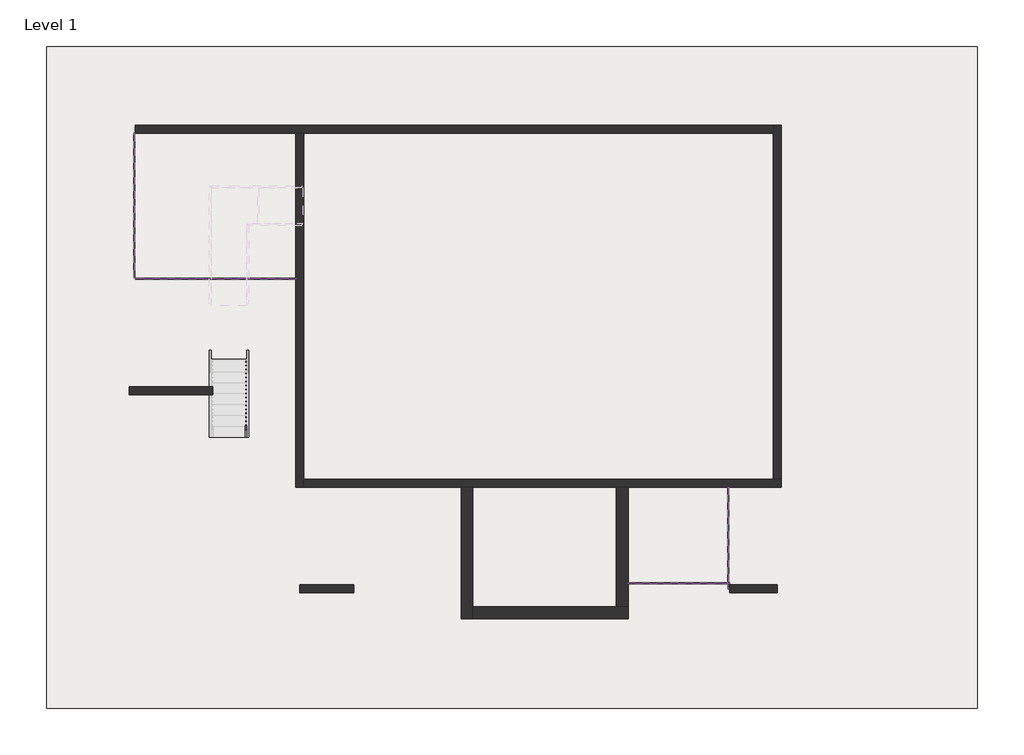
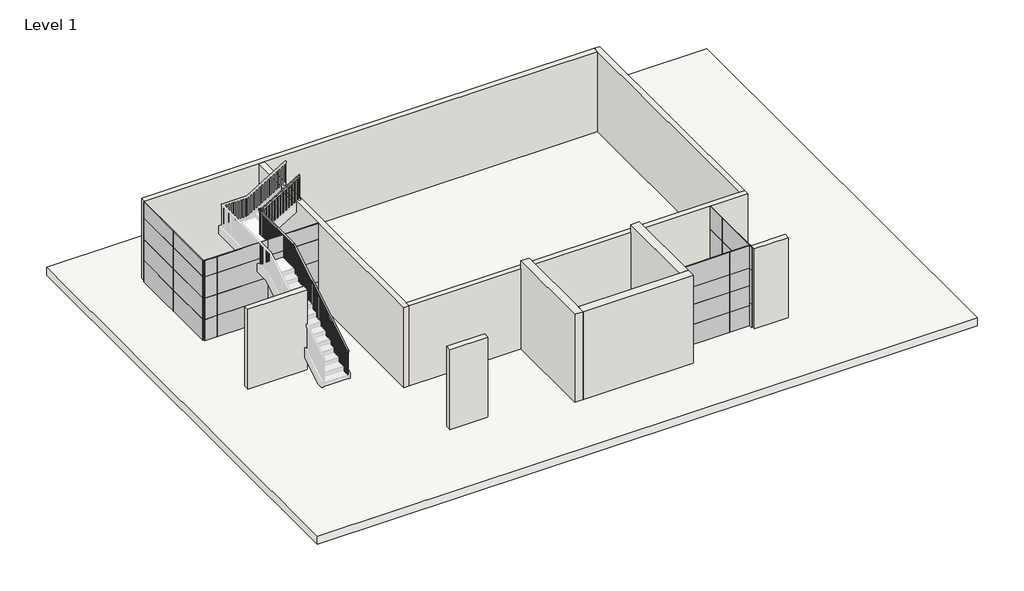
# One storey, part 1 of 2: 38 plates, 10 walls, 1 railing, 1 slab.
"""IFC4 building model written with IfcOpenShell, lengths in millimetres."""

from ifc_helpers import new_model, si_unit, frame, origin, origin_with_axes, place, context, project, spatial, polyline, outline, extrude, faceted_brep, transform, mapped, element, save
from components import system_panel_glazed_6b40402c, system_panel_glazed_10c9008b, system_panel_glazed_62d6a88c, system_panel_glazed_55f8bac4, system_panel_glazed_7c3c2ece, system_panel_glazed_920592d8, system_panel_glazed_22be659e, system_panel_glazed_550407b1, system_panel_glazed_63189bcd, system_panel_glazed_d508e32f, system_panel_glazed_68ef09be, system_panel_glazed_6562854e, system_panel_glazed_2900c437, system_panel_glazed_2cc39d43

model = new_model("IFC4")

# Units and contexts
model_context = context("Model", 3, world=origin())
ifc_project = project(units=[si_unit("LENGTHUNIT", "METRE", prefix="MILLI")], contexts=[model_context])

# Site, building, storey
site = spatial("IfcSite", under=ifc_project)
building = spatial("IfcBuilding", under=site)
storey = spatial("IfcBuildingStorey", under=building, Name="Level 1", Elevation=0.0)

# Plates
placement = place(None, origin())
system_panel_glazed_shape = system_panel_glazed_6b40402c(model_context)
element("IfcPlate", 1, ObjectType="System Panel : Glazed", at=placement, inside=storey, context=model_context, shape_type="MappedRepresentation", body=[
    mapped(system_panel_glazed_shape, transform((4204.5713479, -1055.5434549, 0.0), x_axis=(0.0, 1.0, 0.0), y_axis=(-1.0, 0.0, 0.0), z_axis=(0.0, 0.0, 1.0))),
])
element("IfcPlate", 2, ObjectType="System Panel : Glazed", at=placement, inside=storey, context=model_context, shape_type="MappedRepresentation", body=[
    mapped(system_panel_glazed_shape, transform((4204.5713479, -1055.5434549, 2184.4), x_axis=(0.0, 1.0, 0.0), y_axis=(-1.0, 0.0, 0.0), z_axis=(0.0, 0.0, 1.0))),
])
element("IfcPlate", 3, ObjectType="System Panel : Glazed", at=placement, inside=storey, context=model_context, shape_type="MappedRepresentation", body=[
    mapped(system_panel_glazed_shape, transform((2528.1713479, -1868.3434549, 2184.4), x_axis=(1.0, 0.0, 0.0), y_axis=(0.0, 1.0, 0.0), z_axis=(0.0, 0.0, 1.0))),
])
system_panel_glazed_2_shape = system_panel_glazed_10c9008b(model_context)
element("IfcPlate", 4, ObjectType="System Panel : Glazed", at=placement, inside=storey, context=model_context, shape_type="MappedRepresentation", body=[
    mapped(system_panel_glazed_2_shape, transform((4204.5713479, 239.8565451, 0.0), x_axis=(0.0, 1.0, 0.0), y_axis=(-1.0, 0.0, 0.0), z_axis=(0.0, 0.0, 1.0))),
])
element("IfcPlate", 5, ObjectType="System Panel : Glazed", at=placement, inside=storey, context=model_context, shape_type="MappedRepresentation", body=[
    mapped(system_panel_glazed_2_shape, transform((4204.5713479, 239.8565451, 2184.4), x_axis=(0.0, 1.0, 0.0), y_axis=(-1.0, 0.0, 0.0), z_axis=(0.0, 0.0, 1.0))),
])
element("IfcPlate", 6, ObjectType="System Panel : Glazed", at=placement, inside=storey, context=model_context, shape_type="MappedRepresentation", body=[
    mapped(system_panel_glazed_2_shape, transform((3823.5713479, -1868.3434549, 2184.4), x_axis=(1.0, 0.0, 0.0), y_axis=(0.0, 1.0, 0.0), z_axis=(0.0, 0.0, 1.0))),
])
system_panel_glazed_3_shape = system_panel_glazed_62d6a88c(model_context)
element("IfcPlate", 7, ObjectType="System Panel : Glazed", at=placement, inside=storey, context=model_context, shape_type="MappedRepresentation", body=[
    mapped(system_panel_glazed_3_shape, transform((2528.1713479, -1868.3434549, 1524.0), x_axis=(1.0, 0.0, 0.0), y_axis=(0.0, 1.0, 0.0), z_axis=(0.0, 0.0, 1.0))),
])
system_panel_glazed_4_shape = system_panel_glazed_55f8bac4(model_context)
element("IfcPlate", 8, ObjectType="System Panel : Glazed", at=placement, inside=storey, context=model_context, shape_type="MappedRepresentation", body=[
    mapped(system_panel_glazed_4_shape, transform((3823.5713479, -1868.3434549, 1524.0), x_axis=(1.0, 0.0, 0.0), y_axis=(0.0, 1.0, 0.0), z_axis=(0.0, 0.0, 1.0))),
])
system_panel_glazed_5_shape = system_panel_glazed_7c3c2ece(model_context)
element("IfcPlate", 9, ObjectType="System Panel : Glazed", at=placement, inside=storey, context=model_context, shape_type="MappedRepresentation", body=[
    mapped(system_panel_glazed_5_shape, transform((4204.5713479, -1055.5434549, 863.6), x_axis=(0.0, 1.0, 0.0), y_axis=(-1.0, 0.0, 0.0), z_axis=(0.0, 0.0, 1.0))),
])
system_panel_glazed_6_shape = system_panel_glazed_920592d8(model_context)
element("IfcPlate", 10, ObjectType="System Panel : Glazed", at=placement, inside=storey, context=model_context, shape_type="MappedRepresentation", body=[
    mapped(system_panel_glazed_6_shape, transform((4204.5713479, 239.8565451, 863.6), x_axis=(0.0, 1.0, 0.0), y_axis=(-1.0, 0.0, 0.0), z_axis=(0.0, 0.0, 1.0))),
])
system_panel_glazed_7_shape = system_panel_glazed_22be659e(model_context)
element("IfcPlate", 11, ObjectType="System Panel : Glazed", at=placement, inside=storey, context=model_context, shape_type="MappedRepresentation", body=[
    mapped(system_panel_glazed_7_shape, transform((2528.1713479, -1868.3434549, 0.0), x_axis=(1.0, 0.0, 0.0), y_axis=(0.0, 1.0, 0.0), z_axis=(0.0, 0.0, 1.0))),
])
element("IfcPlate", 12, ObjectType="System Panel : Glazed", at=placement, inside=storey, context=model_context, shape_type="MappedRepresentation", body=[
    mapped(system_panel_glazed_7_shape, transform((2528.1713479, -1868.3434549, 762.0), x_axis=(1.0, 0.0, 0.0), y_axis=(0.0, 1.0, 0.0), z_axis=(0.0, 0.0, 1.0))),
])
system_panel_glazed_8_shape = system_panel_glazed_550407b1(model_context)
element("IfcPlate", 13, ObjectType="System Panel : Glazed", at=placement, inside=storey, context=model_context, shape_type="MappedRepresentation", body=[
    mapped(system_panel_glazed_8_shape, transform((3823.5713479, -1868.3434549, 0.0), x_axis=(1.0, 0.0, 0.0), y_axis=(0.0, 1.0, 0.0), z_axis=(0.0, 0.0, 1.0))),
])
element("IfcPlate", 14, ObjectType="System Panel : Glazed", at=placement, inside=storey, context=model_context, shape_type="MappedRepresentation", body=[
    mapped(system_panel_glazed_8_shape, transform((3823.5713479, -1868.3434549, 762.0), x_axis=(1.0, 0.0, 0.0), y_axis=(0.0, 1.0, 0.0), z_axis=(0.0, 0.0, 1.0))),
])
system_panel_glazed_9_shape = system_panel_glazed_63189bcd(model_context)
element("IfcPlate", 15, ObjectType="System Panel : Glazed", at=placement, inside=storey, context=model_context, shape_type="MappedRepresentation", body=[
    mapped(system_panel_glazed_9_shape, transform((-7784.2286521, 5980.605876, 2438.4), x_axis=(-1.0, 0.0, 0.0), y_axis=(0.0, -1.0, 0.0), z_axis=(0.0, 0.0, 1.0))),
])
element("IfcPlate", 16, ObjectType="System Panel : Glazed", at=placement, inside=storey, context=model_context, shape_type="MappedRepresentation", body=[
    mapped(system_panel_glazed_9_shape, transform((-9613.0286521, 5980.605876, 2438.4), x_axis=(-1.0, 0.0, 0.0), y_axis=(0.0, -1.0, 0.0), z_axis=(0.0, 0.0, 1.0))),
])
element("IfcPlate", 17, ObjectType="System Panel : Glazed", at=placement, inside=storey, context=model_context, shape_type="MappedRepresentation", body=[
    mapped(system_panel_glazed_9_shape, transform((-10970.8984786, 6895.005876, 2438.4), x_axis=(0.0, 1.0, 0.0), y_axis=(-1.0, 0.0, 0.0), z_axis=(0.0, 0.0, 1.0))),
])
element("IfcPlate", 18, ObjectType="System Panel : Glazed", at=placement, inside=storey, context=model_context, shape_type="MappedRepresentation", body=[
    mapped(system_panel_glazed_9_shape, transform((-10970.8984786, 8723.805876, 2438.4), x_axis=(0.0, 1.0, 0.0), y_axis=(-1.0, 0.0, 0.0), z_axis=(0.0, 0.0, 1.0))),
])
system_panel_glazed_10_shape = system_panel_glazed_d508e32f(model_context)
element("IfcPlate", 19, ObjectType="System Panel : Glazed", at=placement, inside=storey, context=model_context, shape_type="MappedRepresentation", body=[
    mapped(system_panel_glazed_10_shape, transform((-10749.1635654, 5980.605876, 2438.4), x_axis=(-1.0, 0.0, 0.0), y_axis=(0.0, -1.0, 0.0), z_axis=(0.0, 0.0, 1.0))),
])
system_panel_glazed_11_shape = system_panel_glazed_68ef09be(model_context)
element("IfcPlate", 20, ObjectType="System Panel : Glazed", at=placement, inside=storey, context=model_context, shape_type="MappedRepresentation", body=[
    mapped(system_panel_glazed_11_shape, transform((-7784.2286521, 5980.605876, 0.0), x_axis=(-1.0, 0.0, 0.0), y_axis=(0.0, -1.0, 0.0), z_axis=(0.0, 0.0, 1.0))),
])
element("IfcPlate", 21, ObjectType="System Panel : Glazed", at=placement, inside=storey, context=model_context, shape_type="MappedRepresentation", body=[
    mapped(system_panel_glazed_11_shape, transform((-10970.8984786, 6895.005876, 0.0), x_axis=(0.0, 1.0, 0.0), y_axis=(-1.0, 0.0, 0.0), z_axis=(0.0, 0.0, 1.0))),
])
element("IfcPlate", 22, ObjectType="System Panel : Glazed", at=placement, inside=storey, context=model_context, shape_type="MappedRepresentation", body=[
    mapped(system_panel_glazed_11_shape, transform((-10970.8984786, 8723.805876, 0.0), x_axis=(0.0, 1.0, 0.0), y_axis=(-1.0, 0.0, 0.0), z_axis=(0.0, 0.0, 1.0))),
])
element("IfcPlate", 23, ObjectType="System Panel : Glazed", at=placement, inside=storey, context=model_context, shape_type="MappedRepresentation", body=[
    mapped(system_panel_glazed_11_shape, transform((-9613.0286521, 5980.605876, 0.0), x_axis=(-1.0, 0.0, 0.0), y_axis=(0.0, -1.0, 0.0), z_axis=(0.0, 0.0, 1.0))),
])
element("IfcPlate", 24, ObjectType="System Panel : Glazed", at=placement, inside=storey, context=model_context, shape_type="MappedRepresentation", body=[
    mapped(system_panel_glazed_11_shape, transform((-7784.2286521, 5980.605876, 1625.6), x_axis=(-1.0, 0.0, 0.0), y_axis=(0.0, -1.0, 0.0), z_axis=(0.0, 0.0, 1.0))),
])
element("IfcPlate", 25, ObjectType="System Panel : Glazed", at=placement, inside=storey, context=model_context, shape_type="MappedRepresentation", body=[
    mapped(system_panel_glazed_11_shape, transform((-9613.0286521, 5980.605876, 1625.6), x_axis=(-1.0, 0.0, 0.0), y_axis=(0.0, -1.0, 0.0), z_axis=(0.0, 0.0, 1.0))),
])
element("IfcPlate", 26, ObjectType="System Panel : Glazed", at=placement, inside=storey, context=model_context, shape_type="MappedRepresentation", body=[
    mapped(system_panel_glazed_11_shape, transform((-7784.2286521, 5980.605876, 812.8), x_axis=(-1.0, 0.0, 0.0), y_axis=(0.0, -1.0, 0.0), z_axis=(0.0, 0.0, 1.0))),
])
element("IfcPlate", 27, ObjectType="System Panel : Glazed", at=placement, inside=storey, context=model_context, shape_type="MappedRepresentation", body=[
    mapped(system_panel_glazed_11_shape, transform((-9613.0286521, 5980.605876, 812.8), x_axis=(-1.0, 0.0, 0.0), y_axis=(0.0, -1.0, 0.0), z_axis=(0.0, 0.0, 1.0))),
])
element("IfcPlate", 28, ObjectType="System Panel : Glazed", at=placement, inside=storey, context=model_context, shape_type="MappedRepresentation", body=[
    mapped(system_panel_glazed_11_shape, transform((-10970.8984786, 6895.005876, 1625.6), x_axis=(0.0, 1.0, 0.0), y_axis=(-1.0, 0.0, 0.0), z_axis=(0.0, 0.0, 1.0))),
])
element("IfcPlate", 29, ObjectType="System Panel : Glazed", at=placement, inside=storey, context=model_context, shape_type="MappedRepresentation", body=[
    mapped(system_panel_glazed_11_shape, transform((-10970.8984786, 8723.805876, 1625.6), x_axis=(0.0, 1.0, 0.0), y_axis=(-1.0, 0.0, 0.0), z_axis=(0.0, 0.0, 1.0))),
])
element("IfcPlate", 30, ObjectType="System Panel : Glazed", at=placement, inside=storey, context=model_context, shape_type="MappedRepresentation", body=[
    mapped(system_panel_glazed_11_shape, transform((-10970.8984786, 6895.005876, 812.8), x_axis=(0.0, 1.0, 0.0), y_axis=(-1.0, 0.0, 0.0), z_axis=(0.0, 0.0, 1.0))),
])
element("IfcPlate", 31, ObjectType="System Panel : Glazed", at=placement, inside=storey, context=model_context, shape_type="MappedRepresentation", body=[
    mapped(system_panel_glazed_11_shape, transform((-10970.8984786, 8723.805876, 812.8), x_axis=(0.0, 1.0, 0.0), y_axis=(-1.0, 0.0, 0.0), z_axis=(0.0, 0.0, 1.0))),
])
system_panel_glazed_12_shape = system_panel_glazed_6562854e(model_context)
element("IfcPlate", 32, ObjectType="System Panel : Glazed", at=placement, inside=storey, context=model_context, shape_type="MappedRepresentation", body=[
    mapped(system_panel_glazed_12_shape, transform((-10749.1635654, 5980.605876, 0.0), x_axis=(-1.0, 0.0, 0.0), y_axis=(0.0, -1.0, 0.0), z_axis=(0.0, 0.0, 1.0))),
])
element("IfcPlate", 33, ObjectType="System Panel : Glazed", at=placement, inside=storey, context=model_context, shape_type="MappedRepresentation", body=[
    mapped(system_panel_glazed_12_shape, transform((-10749.1635654, 5980.605876, 1625.6), x_axis=(-1.0, 0.0, 0.0), y_axis=(0.0, -1.0, 0.0), z_axis=(0.0, 0.0, 1.0))),
])
element("IfcPlate", 34, ObjectType="System Panel : Glazed", at=placement, inside=storey, context=model_context, shape_type="MappedRepresentation", body=[
    mapped(system_panel_glazed_12_shape, transform((-10749.1635654, 5980.605876, 812.8), x_axis=(-1.0, 0.0, 0.0), y_axis=(0.0, -1.0, 0.0), z_axis=(0.0, 0.0, 1.0))),
])
system_panel_glazed_13_shape = system_panel_glazed_2900c437(model_context)
element("IfcPlate", 35, ObjectType="System Panel : Glazed", at=placement, inside=storey, context=model_context, shape_type="MappedRepresentation", body=[
    mapped(system_panel_glazed_13_shape, transform((-10970.8984786, 9650.7312105, 2438.4), x_axis=(0.0, 1.0, 0.0), y_axis=(-1.0, 0.0, 0.0), z_axis=(0.0, 0.0, 1.0))),
])
system_panel_glazed_14_shape = system_panel_glazed_2cc39d43(model_context)
element("IfcPlate", 36, ObjectType="System Panel : Glazed", at=placement, inside=storey, context=model_context, shape_type="MappedRepresentation", body=[
    mapped(system_panel_glazed_14_shape, transform((-10970.8984786, 9650.7312105, 0.0), x_axis=(0.0, 1.0, 0.0), y_axis=(-1.0, 0.0, 0.0), z_axis=(0.0, 0.0, 1.0))),
])
element("IfcPlate", 37, ObjectType="System Panel : Glazed", at=placement, inside=storey, context=model_context, shape_type="MappedRepresentation", body=[
    mapped(system_panel_glazed_14_shape, transform((-10970.8984786, 9650.7312105, 1625.6), x_axis=(0.0, 1.0, 0.0), y_axis=(-1.0, 0.0, 0.0), z_axis=(0.0, 0.0, 1.0))),
])
element("IfcPlate", 38, ObjectType="System Panel : Glazed", at=placement, inside=storey, context=model_context, shape_type="MappedRepresentation", body=[
    mapped(system_panel_glazed_14_shape, transform((-10970.8984786, 9650.7312105, 812.8), x_axis=(0.0, 1.0, 0.0), y_axis=(-1.0, 0.0, 0.0), z_axis=(0.0, 0.0, 1.0))),
])

# Railing
element("IfcRailing", 39, ObjectType="Handrail - Rectangular", at=placement, inside=storey, context=model_context, shape_type="SolidModel", body=[
    faceted_brep([(-8170.6823175, 1898.2635177, 1083.7333333), (-8170.6823175, 1898.2635177, 1024.3318731), (-8119.8823175, 1898.2635177, 1024.3318731), (-8119.8823175, 1898.2635177, 1083.7333333), (-8170.6823175, 5251.0635177, 3115.7333333), (-8170.6823175, 5265.2559271, 3064.9333333), (-8119.8823175, 5265.2559271, 3064.9333333), (-8119.8823175, 5251.0635177, 3115.7333333), (-8170.6823175, 7276.005876, 3115.7333333), (-8170.6823175, 7326.805876, 3064.9333333), (-8119.8823175, 7326.805876, 3064.9333333), (-8119.8823175, 7276.005876, 3115.7333333), (-8170.6823175, 7276.005876, 3161.9151515), (-8170.6823175, 7326.805876, 3111.1151515), (-8119.8823175, 7326.805876, 3111.1151515), (-8119.8823175, 7276.005876, 3161.9151515), (-8170.6823175, 7403.005876, 3161.9151515), (-8170.6823175, 7403.005876, 3111.1151515), (-8119.8823175, 7352.205876, 3111.1151515), (-8119.8823175, 7352.205876, 3161.9151515), (-8043.6823175, 7403.005876, 3161.9151515), (-8029.4899081, 7403.005876, 3111.1151515), (-8029.4899081, 7352.205876, 3111.1151515), (-8043.6823175, 7352.205876, 3161.9151515), (-6722.8823175, 7403.005876, 3962.4), (-6722.8823175, 7352.205876, 3962.4), (-6722.8823175, 7352.205876, 3902.9985397), (-6722.8823175, 7403.005876, 3902.9985397)], [[[0, 1, 2, 3]], [[1, 0, 4, 5]], [[2, 1, 5, 6]], [[3, 2, 6, 7]], [[0, 3, 7, 4]], [[5, 4, 8, 9]], [[6, 5, 9, 10]], [[7, 6, 10, 11]], [[4, 7, 11, 8]], [[9, 8, 12, 13]], [[10, 9, 13, 14]], [[11, 10, 14, 15]], [[8, 11, 15, 12]], [[13, 12, 16, 17]], [[14, 13, 17, 18]], [[15, 14, 18, 19]], [[12, 15, 19, 16]], [[17, 16, 20, 21]], [[18, 17, 21, 22]], [[19, 18, 22, 23]], [[16, 19, 23, 20]], [[24, 25, 26, 27]], [[21, 20, 24, 27]], [[22, 21, 27, 26]], [[23, 22, 26, 25]], [[20, 23, 25, 24]]]),
    extrude(outline(polyline([(3862.5894488, -6789.5573175), (3851.0439943, -6808.6073175), (2878.6666667, -6808.6073175), (2878.6666667, -6789.5573175), (3862.5894488, -6789.5573175)])), frame((0.0, 7368.080876, 0.0), z_axis=(0.0, 1.0, 0.0), x_axis=(0.0, 0.0, 1.0)), (0.0, 0.0, 1.0), 19.05),
    extrude(outline(polyline([(3801.0136913, -6891.1573175), (3789.4682367, -6910.2073175), (2878.6666667, -6910.2073175), (2878.6666667, -6891.1573175), (3801.0136913, -6891.1573175)])), frame((0.0, 7368.080876, 0.0), z_axis=(0.0, 1.0, 0.0), x_axis=(0.0, 0.0, 1.0)), (0.0, 0.0, 1.0), 19.05),
    extrude(outline(polyline([(3739.4379337, -6992.7573175), (3727.8924791, -7011.8073175), (2878.6666667, -7011.8073175), (2878.6666667, -6992.7573175), (3739.4379337, -6992.7573175)])), frame((0.0, 7368.080876, 0.0), z_axis=(0.0, 1.0, 0.0), x_axis=(0.0, 0.0, 1.0)), (0.0, 0.0, 1.0), 19.05),
    extrude(outline(polyline([(3677.8621761, -7094.3573175), (3666.3167216, -7113.4073175), (2709.3333333, -7113.4073175), (2709.3333333, -7094.3573175), (3677.8621761, -7094.3573175)])), frame((0.0, 7368.080876, 0.0), z_axis=(0.0, 1.0, 0.0), x_axis=(0.0, 0.0, 1.0)), (0.0, 0.0, 1.0), 19.05),
    extrude(outline(polyline([(3616.2864185, -7195.9573175), (3604.740964, -7215.0073175), (2709.3333333, -7215.0073175), (2709.3333333, -7195.9573175), (3616.2864185, -7195.9573175)])), frame((0.0, 7368.080876, 0.0), z_axis=(0.0, 1.0, 0.0), x_axis=(0.0, 0.0, 1.0)), (0.0, 0.0, 1.0), 19.05),
    extrude(outline(polyline([(3554.710661, -7297.5573175), (3543.1652064, -7316.6073175), (2540.0, -7316.6073175), (2540.0, -7297.5573175), (3554.710661, -7297.5573175)])), frame((0.0, 7368.080876, 0.0), z_axis=(0.0, 1.0, 0.0), x_axis=(0.0, 0.0, 1.0)), (0.0, 0.0, 1.0), 19.05),
    extrude(outline(polyline([(3493.1349034, -7399.1573175), (3481.5894488, -7418.2073175), (2540.0, -7418.2073175), (2540.0, -7399.1573175), (3493.1349034, -7399.1573175)])), frame((0.0, 7368.080876, 0.0), z_axis=(0.0, 1.0, 0.0), x_axis=(0.0, 0.0, 1.0)), (0.0, 0.0, 1.0), 19.05),
    extrude(outline(polyline([(3431.5591458, -7500.7573175), (3420.0136913, -7519.8073175), (2540.0, -7519.8073175), (2540.0, -7500.7573175), (3431.5591458, -7500.7573175)])), frame((0.0, 7368.080876, 0.0), z_axis=(0.0, 1.0, 0.0), x_axis=(0.0, 0.0, 1.0)), (0.0, 0.0, 1.0), 19.05),
    extrude(outline(polyline([(3369.9833882, -7602.3573175), (3358.4379337, -7621.4073175), (2370.6666667, -7621.4073175), (2370.6666667, -7602.3573175), (3369.9833882, -7602.3573175)])), frame((0.0, 7368.080876, 0.0), z_axis=(0.0, 1.0, 0.0), x_axis=(0.0, 0.0, 1.0)), (0.0, 0.0, 1.0), 19.05),
    extrude(outline(polyline([(3308.4076307, -7703.9573175), (3296.8621761, -7723.0073175), (2370.6666667, -7723.0073175), (2370.6666667, -7703.9573175), (3308.4076307, -7703.9573175)])), frame((0.0, 7368.080876, 0.0), z_axis=(0.0, 1.0, 0.0), x_axis=(0.0, 0.0, 1.0)), (0.0, 0.0, 1.0), 19.05),
    extrude(outline(polyline([(3246.8318731, -7805.5573175), (3235.2864185, -7824.6073175), (2370.6666667, -7824.6073175), (2370.6666667, -7805.5573175), (3246.8318731, -7805.5573175)])), frame((0.0, 7368.080876, 0.0), z_axis=(0.0, 1.0, 0.0), x_axis=(0.0, 0.0, 1.0)), (0.0, 0.0, 1.0), 19.05),
    extrude(outline(polyline([(3185.2561155, -7907.1573175), (3173.710661, -7926.2073175), (2201.3333333, -7926.2073175), (2201.3333333, -7907.1573175), (3185.2561155, -7907.1573175)])), frame((0.0, 7368.080876, 0.0), z_axis=(0.0, 1.0, 0.0), x_axis=(0.0, 0.0, 1.0)), (0.0, 0.0, 1.0), 19.05),
    extrude(outline(polyline([(3123.6803579, -8008.7573175), (3112.1349034, -8027.8073175), (2201.3333333, -8027.8073175), (2201.3333333, -8008.7573175), (3123.6803579, -8008.7573175)])), frame((0.0, 7368.080876, 0.0), z_axis=(0.0, 1.0, 0.0), x_axis=(0.0, 0.0, 1.0)), (0.0, 0.0, 1.0), 19.05),
    extrude(outline(polyline([(-8135.7573175, 7273.5385177), (-8154.8073175, 7273.5385177), (-8154.8073175, 7292.5885177), (-8135.7573175, 7292.5885177), (-8135.7573175, 7273.5385177)])), frame((0.0, 0.0, 2201.3333333), z_axis=(0.0, 0.0, 1.0), x_axis=(1.0, 0.0, 0.0)), (0.0, 0.0, 1.0), 863.6),
    extrude(outline(polyline([(-8135.7573175, 7171.9385177), (-8154.8073175, 7171.9385177), (-8154.8073175, 7190.9885177), (-8135.7573175, 7190.9885177), (-8135.7573175, 7171.9385177)])), frame((0.0, 0.0, 2201.3333333), z_axis=(0.0, 0.0, 1.0), x_axis=(1.0, 0.0, 0.0)), (0.0, 0.0, 1.0), 863.6),
    extrude(outline(polyline([(-8135.7573175, 7070.3385177), (-8154.8073175, 7070.3385177), (-8154.8073175, 7089.3885177), (-8135.7573175, 7089.3885177), (-8135.7573175, 7070.3385177)])), frame((0.0, 0.0, 2201.3333333), z_axis=(0.0, 0.0, 1.0), x_axis=(1.0, 0.0, 0.0)), (0.0, 0.0, 1.0), 863.6),
    extrude(outline(polyline([(-8135.7573175, 6968.7385177), (-8154.8073175, 6968.7385177), (-8154.8073175, 6987.7885177), (-8135.7573175, 6987.7885177), (-8135.7573175, 6968.7385177)])), frame((0.0, 0.0, 2201.3333333), z_axis=(0.0, 0.0, 1.0), x_axis=(1.0, 0.0, 0.0)), (0.0, 0.0, 1.0), 863.6),
    extrude(outline(polyline([(-8135.7573175, 6867.1385177), (-8154.8073175, 6867.1385177), (-8154.8073175, 6886.1885177), (-8135.7573175, 6886.1885177), (-8135.7573175, 6867.1385177)])), frame((0.0, 0.0, 2201.3333333), z_axis=(0.0, 0.0, 1.0), x_axis=(1.0, 0.0, 0.0)), (0.0, 0.0, 1.0), 863.6),
    extrude(outline(polyline([(-8135.7573175, 6765.5385177), (-8154.8073175, 6765.5385177), (-8154.8073175, 6784.5885177), (-8135.7573175, 6784.5885177), (-8135.7573175, 6765.5385177)])), frame((0.0, 0.0, 2201.3333333), z_axis=(0.0, 0.0, 1.0), x_axis=(1.0, 0.0, 0.0)), (0.0, 0.0, 1.0), 863.6),
    extrude(outline(polyline([(-8135.7573175, 6663.9385177), (-8154.8073175, 6663.9385177), (-8154.8073175, 6682.9885177), (-8135.7573175, 6682.9885177), (-8135.7573175, 6663.9385177)])), frame((0.0, 0.0, 2201.3333333), z_axis=(0.0, 0.0, 1.0), x_axis=(1.0, 0.0, 0.0)), (0.0, 0.0, 1.0), 863.6),
    extrude(outline(polyline([(-8135.7573175, 6562.3385177), (-8154.8073175, 6562.3385177), (-8154.8073175, 6581.3885177), (-8135.7573175, 6581.3885177), (-8135.7573175, 6562.3385177)])), frame((0.0, 0.0, 2201.3333333), z_axis=(0.0, 0.0, 1.0), x_axis=(1.0, 0.0, 0.0)), (0.0, 0.0, 1.0), 863.6),
    extrude(outline(polyline([(-8135.7573175, 6460.7385177), (-8154.8073175, 6460.7385177), (-8154.8073175, 6479.7885177), (-8135.7573175, 6479.7885177), (-8135.7573175, 6460.7385177)])), frame((0.0, 0.0, 2201.3333333), z_axis=(0.0, 0.0, 1.0), x_axis=(1.0, 0.0, 0.0)), (0.0, 0.0, 1.0), 863.6),
    extrude(outline(polyline([(-8135.7573175, 6359.1385177), (-8154.8073175, 6359.1385177), (-8154.8073175, 6378.1885177), (-8135.7573175, 6378.1885177), (-8135.7573175, 6359.1385177)])), frame((0.0, 0.0, 2201.3333333), z_axis=(0.0, 0.0, 1.0), x_axis=(1.0, 0.0, 0.0)), (0.0, 0.0, 1.0), 863.6),
    extrude(outline(polyline([(-8135.7573175, 6257.5385177), (-8154.8073175, 6257.5385177), (-8154.8073175, 6276.5885177), (-8135.7573175, 6276.5885177), (-8135.7573175, 6257.5385177)])), frame((0.0, 0.0, 2201.3333333), z_axis=(0.0, 0.0, 1.0), x_axis=(1.0, 0.0, 0.0)), (0.0, 0.0, 1.0), 863.6),
    extrude(outline(polyline([(-8135.7573175, 6155.9385177), (-8154.8073175, 6155.9385177), (-8154.8073175, 6174.9885177), (-8135.7573175, 6174.9885177), (-8135.7573175, 6155.9385177)])), frame((0.0, 0.0, 2201.3333333), z_axis=(0.0, 0.0, 1.0), x_axis=(1.0, 0.0, 0.0)), (0.0, 0.0, 1.0), 863.6),
    extrude(outline(polyline([(-8135.7573175, 6054.3385177), (-8154.8073175, 6054.3385177), (-8154.8073175, 6073.3885177), (-8135.7573175, 6073.3885177), (-8135.7573175, 6054.3385177)])), frame((0.0, 0.0, 2201.3333333), z_axis=(0.0, 0.0, 1.0), x_axis=(1.0, 0.0, 0.0)), (0.0, 0.0, 1.0), 863.6),
    extrude(outline(polyline([(-8135.7573175, 5952.7385177), (-8154.8073175, 5952.7385177), (-8154.8073175, 5971.7885177), (-8135.7573175, 5971.7885177), (-8135.7573175, 5952.7385177)])), frame((0.0, 0.0, 2201.3333333), z_axis=(0.0, 0.0, 1.0), x_axis=(1.0, 0.0, 0.0)), (0.0, 0.0, 1.0), 863.6),
    extrude(outline(polyline([(-8135.7573175, 5851.1385177), (-8154.8073175, 5851.1385177), (-8154.8073175, 5870.1885177), (-8135.7573175, 5870.1885177), (-8135.7573175, 5851.1385177)])), frame((0.0, 0.0, 2201.3333333), z_axis=(0.0, 0.0, 1.0), x_axis=(1.0, 0.0, 0.0)), (0.0, 0.0, 1.0), 863.6),
    extrude(outline(polyline([(-8135.7573175, 5749.5385177), (-8154.8073175, 5749.5385177), (-8154.8073175, 5768.5885177), (-8135.7573175, 5768.5885177), (-8135.7573175, 5749.5385177)])), frame((0.0, 0.0, 2201.3333333), z_axis=(0.0, 0.0, 1.0), x_axis=(1.0, 0.0, 0.0)), (0.0, 0.0, 1.0), 863.6),
    extrude(outline(polyline([(-8135.7573175, 5647.9385177), (-8154.8073175, 5647.9385177), (-8154.8073175, 5666.9885177), (-8135.7573175, 5666.9885177), (-8135.7573175, 5647.9385177)])), frame((0.0, 0.0, 2201.3333333), z_axis=(0.0, 0.0, 1.0), x_axis=(1.0, 0.0, 0.0)), (0.0, 0.0, 1.0), 863.6),
    extrude(outline(polyline([(-8135.7573175, 5546.3385177), (-8154.8073175, 5546.3385177), (-8154.8073175, 5565.3885177), (-8135.7573175, 5565.3885177), (-8135.7573175, 5546.3385177)])), frame((0.0, 0.0, 2201.3333333), z_axis=(0.0, 0.0, 1.0), x_axis=(1.0, 0.0, 0.0)), (0.0, 0.0, 1.0), 863.6),
    extrude(outline(polyline([(-8135.7573175, 5444.7385177), (-8154.8073175, 5444.7385177), (-8154.8073175, 5463.7885177), (-8135.7573175, 5463.7885177), (-8135.7573175, 5444.7385177)])), frame((0.0, 0.0, 2201.3333333), z_axis=(0.0, 0.0, 1.0), x_axis=(1.0, 0.0, 0.0)), (0.0, 0.0, 1.0), 863.6),
    extrude(outline(polyline([(-8135.7573175, 5343.1385177), (-8154.8073175, 5343.1385177), (-8154.8073175, 5362.1885177), (-8135.7573175, 5362.1885177), (-8135.7573175, 5343.1385177)])), frame((0.0, 0.0, 2201.3333333), z_axis=(0.0, 0.0, 1.0), x_axis=(1.0, 0.0, 0.0)), (0.0, 0.0, 1.0), 863.6),
    extrude(outline(polyline([(5139.9385177, 2988.9833882), (5158.9885177, 3000.5288428), (5158.9885177, 2032.0), (5139.9385177, 2032.0), (5139.9385177, 2988.9833882)])), frame((-8154.8073175, 0.0, 0.0), z_axis=(1.0, 0.0, 0.0), x_axis=(0.0, 1.0, 0.0)), (0.0, 0.0, 1.0), 19.05),
    extrude(outline(polyline([(5038.3385177, 2927.4076307), (5057.3885177, 2938.9530852), (5057.3885177, 2032.0), (5038.3385177, 2032.0), (5038.3385177, 2927.4076307)])), frame((-8154.8073175, 0.0, 0.0), z_axis=(1.0, 0.0, 0.0), x_axis=(0.0, 1.0, 0.0)), (0.0, 0.0, 1.0), 19.05),
    extrude(outline(polyline([(4936.7385177, 2865.8318731), (4955.7885177, 2877.3773276), (4955.7885177, 1862.6666667), (4936.7385177, 1862.6666667), (4936.7385177, 2865.8318731)])), frame((-8154.8073175, 0.0, 0.0), z_axis=(1.0, 0.0, 0.0), x_axis=(0.0, 1.0, 0.0)), (0.0, 0.0, 1.0), 19.05),
    extrude(outline(polyline([(4835.1385177, 2804.2561155), (4854.1885177, 2815.80157), (4854.1885177, 1862.6666667), (4835.1385177, 1862.6666667), (4835.1385177, 2804.2561155)])), frame((-8154.8073175, 0.0, 0.0), z_axis=(1.0, 0.0, 0.0), x_axis=(0.0, 1.0, 0.0)), (0.0, 0.0, 1.0), 19.05),
    extrude(outline(polyline([(4733.5385177, 2742.6803579), (4752.5885177, 2754.2258125), (4752.5885177, 1862.6666667), (4733.5385177, 1862.6666667), (4733.5385177, 2742.6803579)])), frame((-8154.8073175, 0.0, 0.0), z_axis=(1.0, 0.0, 0.0), x_axis=(0.0, 1.0, 0.0)), (0.0, 0.0, 1.0), 19.05),
    extrude(outline(polyline([(4631.9385177, 2681.1046004), (4650.9885177, 2692.6500549), (4650.9885177, 1693.3333333), (4631.9385177, 1693.3333333), (4631.9385177, 2681.1046004)])), frame((-8154.8073175, 0.0, 0.0), z_axis=(1.0, 0.0, 0.0), x_axis=(0.0, 1.0, 0.0)), (0.0, 0.0, 1.0), 19.05),
    extrude(outline(polyline([(4530.3385177, 2619.5288428), (4549.3885177, 2631.0742973), (4549.3885177, 1693.3333333), (4530.3385177, 1693.3333333), (4530.3385177, 2619.5288428)])), frame((-8154.8073175, 0.0, 0.0), z_axis=(1.0, 0.0, 0.0), x_axis=(0.0, 1.0, 0.0)), (0.0, 0.0, 1.0), 19.05),
    extrude(outline(polyline([(4428.7385177, 2557.9530852), (4447.7885177, 2569.4985397), (4447.7885177, 1693.3333333), (4428.7385177, 1693.3333333), (4428.7385177, 2557.9530852)])), frame((-8154.8073175, 0.0, 0.0), z_axis=(1.0, 0.0, 0.0), x_axis=(0.0, 1.0, 0.0)), (0.0, 0.0, 1.0), 19.05),
    extrude(outline(polyline([(4327.1385177, 2496.3773276), (4346.1885177, 2507.9227822), (4346.1885177, 1524.0), (4327.1385177, 1524.0), (4327.1385177, 2496.3773276)])), frame((-8154.8073175, 0.0, 0.0), z_axis=(1.0, 0.0, 0.0), x_axis=(0.0, 1.0, 0.0)), (0.0, 0.0, 1.0), 19.05),
    extrude(outline(polyline([(4225.5385177, 2434.80157), (4244.5885177, 2446.3470246), (4244.5885177, 1524.0), (4225.5385177, 1524.0), (4225.5385177, 2434.80157)])), frame((-8154.8073175, 0.0, 0.0), z_axis=(1.0, 0.0, 0.0), x_axis=(0.0, 1.0, 0.0)), (0.0, 0.0, 1.0), 19.05),
    extrude(outline(polyline([(4123.9385177, 2373.2258125), (4142.9885177, 2384.771267), (4142.9885177, 1524.0), (4123.9385177, 1524.0), (4123.9385177, 2373.2258125)])), frame((-8154.8073175, 0.0, 0.0), z_axis=(1.0, 0.0, 0.0), x_axis=(0.0, 1.0, 0.0)), (0.0, 0.0, 1.0), 19.05),
    extrude(outline(polyline([(4022.3385177, 2311.6500549), (4041.3885177, 2323.1955094), (4041.3885177, 1354.6666667), (4022.3385177, 1354.6666667), (4022.3385177, 2311.6500549)])), frame((-8154.8073175, 0.0, 0.0), z_axis=(1.0, 0.0, 0.0), x_axis=(0.0, 1.0, 0.0)), (0.0, 0.0, 1.0), 19.05),
    extrude(outline(polyline([(3920.7385177, 2250.0742973), (3939.7885177, 2261.6197519), (3939.7885177, 1354.6666667), (3920.7385177, 1354.6666667), (3920.7385177, 2250.0742973)])), frame((-8154.8073175, 0.0, 0.0), z_axis=(1.0, 0.0, 0.0), x_axis=(0.0, 1.0, 0.0)), (0.0, 0.0, 1.0), 19.05),
    extrude(outline(polyline([(3819.1385177, 2188.4985397), (3838.1885177, 2200.0439943), (3838.1885177, 1185.3333333), (3819.1385177, 1185.3333333), (3819.1385177, 2188.4985397)])), frame((-8154.8073175, 0.0, 0.0), z_axis=(1.0, 0.0, 0.0), x_axis=(0.0, 1.0, 0.0)), (0.0, 0.0, 1.0), 19.05),
    extrude(outline(polyline([(3717.5385177, 2126.9227822), (3736.5885177, 2138.4682367), (3736.5885177, 1185.3333333), (3717.5385177, 1185.3333333), (3717.5385177, 2126.9227822)])), frame((-8154.8073175, 0.0, 0.0), z_axis=(1.0, 0.0, 0.0), x_axis=(0.0, 1.0, 0.0)), (0.0, 0.0, 1.0), 19.05),
    extrude(outline(polyline([(3615.9385177, 2065.3470246), (3634.9885177, 2076.8924791), (3634.9885177, 1185.3333333), (3615.9385177, 1185.3333333), (3615.9385177, 2065.3470246)])), frame((-8154.8073175, 0.0, 0.0), z_axis=(1.0, 0.0, 0.0), x_axis=(0.0, 1.0, 0.0)), (0.0, 0.0, 1.0), 19.05),
    extrude(outline(polyline([(3514.3385177, 2003.771267), (3533.3885177, 2015.3167216), (3533.3885177, 1016.0), (3514.3385177, 1016.0), (3514.3385177, 2003.771267)])), frame((-8154.8073175, 0.0, 0.0), z_axis=(1.0, 0.0, 0.0), x_axis=(0.0, 1.0, 0.0)), (0.0, 0.0, 1.0), 19.05),
    extrude(outline(polyline([(3412.7385177, 1942.1955094), (3431.7885177, 1953.740964), (3431.7885177, 1016.0), (3412.7385177, 1016.0), (3412.7385177, 1942.1955094)])), frame((-8154.8073175, 0.0, 0.0), z_axis=(1.0, 0.0, 0.0), x_axis=(0.0, 1.0, 0.0)), (0.0, 0.0, 1.0), 19.05),
    extrude(outline(polyline([(3311.1385177, 1880.6197519), (3330.1885177, 1892.1652064), (3330.1885177, 1016.0), (3311.1385177, 1016.0), (3311.1385177, 1880.6197519)])), frame((-8154.8073175, 0.0, 0.0), z_axis=(1.0, 0.0, 0.0), x_axis=(0.0, 1.0, 0.0)), (0.0, 0.0, 1.0), 19.05),
    extrude(outline(polyline([(3209.5385177, 1819.0439943), (3228.5885177, 1830.5894488), (3228.5885177, 846.6666667), (3209.5385177, 846.6666667), (3209.5385177, 1819.0439943)])), frame((-8154.8073175, 0.0, 0.0), z_axis=(1.0, 0.0, 0.0), x_axis=(0.0, 1.0, 0.0)), (0.0, 0.0, 1.0), 19.05),
    extrude(outline(polyline([(3107.9385177, 1757.4682367), (3126.9885177, 1769.0136913), (3126.9885177, 846.6666667), (3107.9385177, 846.6666667), (3107.9385177, 1757.4682367)])), frame((-8154.8073175, 0.0, 0.0), z_axis=(1.0, 0.0, 0.0), x_axis=(0.0, 1.0, 0.0)), (0.0, 0.0, 1.0), 19.05),
    extrude(outline(polyline([(3006.3385177, 1695.8924791), (3025.3885177, 1707.4379337), (3025.3885177, 846.6666667), (3006.3385177, 846.6666667), (3006.3385177, 1695.8924791)])), frame((-8154.8073175, 0.0, 0.0), z_axis=(1.0, 0.0, 0.0), x_axis=(0.0, 1.0, 0.0)), (0.0, 0.0, 1.0), 19.05),
    extrude(outline(polyline([(2904.7385177, 1634.3167216), (2923.7885177, 1645.8621761), (2923.7885177, 677.3333333), (2904.7385177, 677.3333333), (2904.7385177, 1634.3167216)])), frame((-8154.8073175, 0.0, 0.0), z_axis=(1.0, 0.0, 0.0), x_axis=(0.0, 1.0, 0.0)), (0.0, 0.0, 1.0), 19.05),
    extrude(outline(polyline([(2803.1385177, 1572.740964), (2822.1885177, 1584.2864185), (2822.1885177, 677.3333333), (2803.1385177, 677.3333333), (2803.1385177, 1572.740964)])), frame((-8154.8073175, 0.0, 0.0), z_axis=(1.0, 0.0, 0.0), x_axis=(0.0, 1.0, 0.0)), (0.0, 0.0, 1.0), 19.05),
    extrude(outline(polyline([(2701.5385177, 1511.1652064), (2720.5885177, 1522.710661), (2720.5885177, 508.0), (2701.5385177, 508.0), (2701.5385177, 1511.1652064)])), frame((-8154.8073175, 0.0, 0.0), z_axis=(1.0, 0.0, 0.0), x_axis=(0.0, 1.0, 0.0)), (0.0, 0.0, 1.0), 19.05),
    extrude(outline(polyline([(2599.9385177, 1449.5894488), (2618.9885177, 1461.1349034), (2618.9885177, 508.0), (2599.9385177, 508.0), (2599.9385177, 1449.5894488)])), frame((-8154.8073175, 0.0, 0.0), z_axis=(1.0, 0.0, 0.0), x_axis=(0.0, 1.0, 0.0)), (0.0, 0.0, 1.0), 19.05),
    extrude(outline(polyline([(2498.3385177, 1388.0136913), (2517.3885177, 1399.5591458), (2517.3885177, 508.0), (2498.3385177, 508.0), (2498.3385177, 1388.0136913)])), frame((-8154.8073175, 0.0, 0.0), z_axis=(1.0, 0.0, 0.0), x_axis=(0.0, 1.0, 0.0)), (0.0, 0.0, 1.0), 19.05),
    extrude(outline(polyline([(2396.7385177, 1326.4379337), (2415.7885177, 1337.9833882), (2415.7885177, 338.6666667), (2396.7385177, 338.6666667), (2396.7385177, 1326.4379337)])), frame((-8154.8073175, 0.0, 0.0), z_axis=(1.0, 0.0, 0.0), x_axis=(0.0, 1.0, 0.0)), (0.0, 0.0, 1.0), 19.05),
    extrude(outline(polyline([(2295.1385177, 1264.8621761), (2314.1885177, 1276.4076307), (2314.1885177, 338.6666667), (2295.1385177, 338.6666667), (2295.1385177, 1264.8621761)])), frame((-8154.8073175, 0.0, 0.0), z_axis=(1.0, 0.0, 0.0), x_axis=(0.0, 1.0, 0.0)), (0.0, 0.0, 1.0), 19.05),
    extrude(outline(polyline([(2193.5385177, 1203.2864185), (2212.5885177, 1214.8318731), (2212.5885177, 338.6666667), (2193.5385177, 338.6666667), (2193.5385177, 1203.2864185)])), frame((-8154.8073175, 0.0, 0.0), z_axis=(1.0, 0.0, 0.0), x_axis=(0.0, 1.0, 0.0)), (0.0, 0.0, 1.0), 19.05),
    extrude(outline(polyline([(2091.9385177, 1141.710661), (2110.9885177, 1153.2561155), (2110.9885177, 169.3333333), (2091.9385177, 169.3333333), (2091.9385177, 1141.710661)])), frame((-8154.8073175, 0.0, 0.0), z_axis=(1.0, 0.0, 0.0), x_axis=(0.0, 1.0, 0.0)), (0.0, 0.0, 1.0), 19.05),
    extrude(outline(polyline([(1990.3385177, 1080.1349034), (2009.3885177, 1091.6803579), (2009.3885177, 169.3333333), (1990.3385177, 169.3333333), (1990.3385177, 1080.1349034)])), frame((-8154.8073175, 0.0, 0.0), z_axis=(1.0, 0.0, 0.0), x_axis=(0.0, 1.0, 0.0)), (0.0, 0.0, 1.0), 19.05),
    extrude(outline(polyline([(-8129.4073175, 7368.080876), (-8129.4073175, 7387.130876), (-8110.3573175, 7387.130876), (-8110.3573175, 7368.080876), (-8129.4073175, 7368.080876)])), frame((0.0, 0.0, 2201.3333333), z_axis=(0.0, 0.0, 1.0), x_axis=(1.0, 0.0, 0.0)), (0.0, 0.0, 1.0), 909.7818182),
    extrude(outline(polyline([(-8135.7573175, 7368.080876), (-8154.8073175, 7368.080876), (-8154.8073175, 7387.130876), (-8135.7573175, 7387.130876), (-8135.7573175, 7368.080876)])), frame((0.0, 0.0, 2201.3333333), z_axis=(0.0, 0.0, 1.0), x_axis=(1.0, 0.0, 0.0)), (0.0, 0.0, 1.0), 909.7818182),
    extrude(outline(polyline([(5241.5385177, 3050.5591458), (5260.5885177, 3062.1046004), (5260.5885177, 2201.3333333), (5241.5385177, 2201.3333333), (5241.5385177, 3050.5591458)])), frame((-8154.8073175, 0.0, 0.0), z_axis=(1.0, 0.0, 0.0), x_axis=(0.0, 1.0, 0.0)), (0.0, 0.0, 1.0), 19.05),
    extrude(outline(polyline([(3902.9985397, -6722.8823175), (3891.4530852, -6741.9323175), (2878.6666667, -6741.9323175), (2878.6666667, -6722.8823175), (3902.9985397, -6722.8823175)])), frame((0.0, 7368.080876, 0.0), z_axis=(0.0, 1.0, 0.0), x_axis=(0.0, 0.0, 1.0)), (0.0, 0.0, 1.0), 19.05),
    extrude(outline(polyline([(1898.2635177, 1024.3318731), (1917.3135177, 1035.8773276), (1917.3135177, 169.3333333), (1898.2635177, 169.3333333), (1898.2635177, 1024.3318731)])), frame((-8154.8073175, 0.0, 0.0), z_axis=(1.0, 0.0, 0.0), x_axis=(0.0, 1.0, 0.0)), (0.0, 0.0, 1.0), 19.05),
])

# Slab
element("IfcSlab", 40, ObjectType="Generic - 12\" 2", at=placement, inside=storey, context=model_context, shape_type="SweptSolid", body=[
    extrude(outline(polyline([(10535.3901868, 11876.024998), (10535.3901868, -5017.9434549), (-13239.0098132, -5017.9434549), (-13239.0098132, 11876.024998), (10535.3901868, 11876.024998)])), frame((0.0, 0.0, -304.8), z_axis=(0.0, 0.0, 1.0), x_axis=(1.0, 0.0, 0.0)), (0.0, 0.0, 1.0), 304.8),
])

# Walls
element("IfcWall", 41, ObjectType="Generic - 12\"", at=placement, inside=storey, context=model_context, shape_type="Brep", body=[
    faceted_brep([(-2653.4286521, 620.8565451, 0.0), (-2653.4286521, -2731.9434549, 0.0), (-2653.4286521, -2731.9434549, 3352.8), (-2653.4286521, 620.8565451, 3352.8), (-2348.6286521, 620.8565451, 0.0), (-2348.6286521, 620.8565451, 3352.8), (-2348.6286521, -2427.1434549, 3352.8), (-2348.6286521, -2731.9434549, 3352.8), (-2348.6286521, -2731.9434549, 0.0), (-2348.6286521, -2427.1434549, 0.0)], [[[0, 1, 2, 3]], [[4, 5, 6, 7, 8, 9]], [[1, 0, 4, 9, 8]], [[3, 2, 7, 6, 5]], [[0, 3, 5, 4]], [[2, 1, 8, 7]]]),
])
element("IfcWall", 42, ObjectType="Generic - 12\"", at=placement, inside=storey, context=model_context, shape_type="Brep", body=[
    faceted_brep([(-2348.6286521, -2731.9434549, 0.0), (1613.7713479, -2731.9434549, 0.0), (1613.7713479, -2731.9434549, 3352.8), (-2348.6286521, -2731.9434549, 3352.8), (-2348.6286521, -2427.1434549, 0.0), (-2348.6286521, -2427.1434549, 3352.8), (1308.9713479, -2427.1434549, 3352.8), (1613.7713479, -2427.1434549, 3352.8), (1613.7713479, -2427.1434549, 0.0), (1308.9713479, -2427.1434549, 0.0)], [[[0, 1, 2, 3]], [[4, 5, 6, 7, 8, 9]], [[1, 0, 4, 9, 8]], [[3, 2, 7, 6, 5]], [[0, 3, 5, 4]], [[2, 1, 8, 7]]]),
])
element("IfcWall", 43, ObjectType="Generic - 12\"", at=placement, inside=storey, context=model_context, shape_type="SweptSolid", body=[
    extrude(outline(polyline([(1613.7713479, 620.8565451), (1613.7713479, -2427.1434549), (1308.9713479, -2427.1434549), (1308.9713479, 620.8565451), (1613.7713479, 620.8565451)])), origin_with_axes(), (0.0, 0.0, 1.0), 3352.8),
])
element("IfcWall", 44, ObjectType="Generic - 8\" 2", at=placement, inside=storey, context=model_context, shape_type="Brep", body=[
    faceted_brep([(-10970.8984786, 9663.2565451, 0.0), (-6869.8286521, 9663.2565451, 0.0), (-6666.6286521, 9663.2565451, 0.0), (5322.1713479, 9663.2565451, 0.0), (5322.1713479, 9663.2565451, 3048.0), (-6666.6286521, 9663.2565451, 3048.0), (-6869.8286521, 9663.2565451, 3048.0), (-10970.8984786, 9663.2565451, 3048.0), (-10970.8984786, 9866.4565451, 0.0), (-10970.8984786, 9866.4565451, 3048.0), (5322.1713479, 9866.4565451, 3048.0), (5322.1713479, 9866.4565451, 0.0)], [[[0, 1, 2, 3, 4, 5, 6, 7]], [[8, 9, 10, 11]], [[3, 2, 1, 0, 8, 11]], [[7, 6, 5, 4, 10, 9]], [[0, 7, 9, 8]], [[4, 3, 11, 10]]]),
])
element("IfcWall", 45, ObjectType="Generic - 8\" 2", at=placement, inside=storey, context=model_context, shape_type="Brep", body=[
    faceted_brep([(-6666.6286521, 620.8565451, 0.0), (-6666.6286521, 824.0565451, 0.0), (-6666.6286521, 9663.2565451, 0.0), (-6666.6286521, 9663.2565451, 3048.0), (-6666.6286521, 824.0565451, 3048.0), (-6666.6286521, 620.8565451, 3048.0), (-6869.8286521, 620.8565451, 0.0), (-6869.8286521, 620.8565451, 3048.0), (-6869.8286521, 9663.2565451, 3048.0), (-6869.8286521, 9663.2565451, 0.0)], [[[0, 1, 2, 3, 4, 5]], [[6, 7, 8, 9]], [[2, 1, 0, 6, 9]], [[5, 4, 3, 8, 7]], [[0, 5, 7, 6]], [[3, 2, 9, 8]]]),
])
element("IfcWall", 46, ObjectType="Generic - 8\" 2", at=placement, inside=storey, context=model_context, shape_type="Brep", body=[
    faceted_brep([(5525.3713479, 824.0565451, 0.0), (5322.1713479, 824.0565451, 0.0), (-6666.6286521, 824.0565451, 0.0), (-6666.6286521, 824.0565451, 3048.0), (5322.1713479, 824.0565451, 3048.0), (5525.3713479, 824.0565451, 3048.0), (5525.3713479, 620.8565451, 0.0), (5525.3713479, 620.8565451, 3048.0), (-6666.6286521, 620.8565451, 3048.0), (-6666.6286521, 620.8565451, 0.0), (-2653.4286521, 620.8565451, 0.0), (-2348.6286521, 620.8565451, 0.0), (1308.9713479, 620.8565451, 0.0), (1613.7713479, 620.8565451, 0.0)], [[[0, 1, 2, 3, 4, 5]], [[6, 7, 8, 9, 10, 11, 12, 13]], [[2, 1, 0, 6, 13, 12, 11, 10, 9]], [[5, 4, 3, 8, 7]], [[0, 5, 7, 6]], [[3, 2, 9, 8]]]),
])
element("IfcWall", 47, ObjectType="Generic - 8\" 2", at=placement, inside=storey, context=model_context, shape_type="Brep", body=[
    faceted_brep([(5322.1713479, 9866.4565451, 0.0), (5322.1713479, 9663.2565451, 0.0), (5322.1713479, 824.0565451, 0.0), (5322.1713479, 824.0565451, 3048.0), (5322.1713479, 9663.2565451, 3048.0), (5322.1713479, 9866.4565451, 3048.0), (5525.3713479, 9866.4565451, 0.0), (5525.3713479, 9866.4565451, 3048.0), (5525.3713479, 824.0565451, 3048.0), (5525.3713479, 824.0565451, 0.0)], [[[0, 1, 2, 3, 4, 5]], [[6, 7, 8, 9]], [[2, 1, 0, 6, 9]], [[5, 4, 3, 8, 7]], [[0, 5, 7, 6]], [[3, 2, 9, 8]]]),
])
element("IfcWall", 48, ObjectType="Generic - 8\" 2", at=placement, inside=storey, context=model_context, shape_type="SweptSolid", body=[
    extrude(outline(polyline([(-6768.2286521, -1868.3434549), (-5396.6286521, -1868.3434549), (-5396.6286521, -2071.5434549), (-6768.2286521, -2071.5434549), (-6768.2286521, -1868.3434549)])), origin_with_axes(), (0.0, 0.0, 1.0), 3048.0),
])
element("IfcWall", 49, ObjectType="Generic - 8\" 2", at=placement, inside=storey, context=model_context, shape_type="SweptSolid", body=[
    extrude(outline(polyline([(5423.7713479, -2071.5434549), (4204.5713479, -2071.5434549), (4204.5713479, -1868.3434549), (5423.7713479, -1868.3434549), (5423.7713479, -2071.5434549)])), origin_with_axes(), (0.0, 0.0, 1.0), 3048.0),
])
element("IfcWall", 50, ObjectType="Generic - 8\" 3", at=placement, inside=storey, context=model_context, shape_type="SweptSolid", body=[
    extrude(outline(polyline([(-11123.2984786, 3186.605876), (-8989.6984786, 3186.605876), (-8989.6984786, 2983.405876), (-11123.2984786, 2983.405876), (-11123.2984786, 3186.605876)])), origin_with_axes(), (0.0, 0.0, 1.0), 3048.0),
])

save(model, "model.ifc")

# Revit data of these elements
# Type "System Panel : Glazed"
#   Construction Type Id = "GSP4R"
#   Analytic Construction = "1/8 in Pilkington single glazing"
#   Visual Light Transmittance = 0.9
#   Solar Heat Gain Coefficient = 0.86
#   Heat Transfer Coefficient (U) = 1.18115 BTU/(h·ft²·°F)
# Type "Handrail - Rectangular"
#   Assembly Code = "C2010400"
#   built-in parameter 1008612 = 0.0416667 (stored number, unit not read)
#   built-in parameter 1008611 = 0.0416667 (stored number, unit not read)
#   built-in parameter 1008609 = 0.333333 (stored number, unit not read)
#   built-in parameter 1008604 = 0.166667 (stored number, unit not read)
#   built-in parameter 1008603 = 0.166667 (stored number, unit not read)
#   Railing Height = 3' - 0"
#   built-in parameter 1008630 = 2
#   built-in parameter 1008610 = 2
#   built-in parameter 1008618 = Baluster - Square : 3/4"
# Type "Generic - 12\" 2"
#   Assembly Code = "B1010"
#   Function = 0
#   Layers, outside or top first: 1' - 0" "Acoustic Ceiling Tile 24 x 24" (function 1)
# Type "Generic - 12\""
#   Assembly Code = "B2010"
#   Layers, outside or top first: 1' - 0" "Laminate, Ivory, Matte" (function 1)
# Type "Generic - 8\" 2"
#   Assembly Code = "B2010"
#   Layers, outside or top first: 0' - 8" "Acoustic Ceiling Tile 24 x 24" (function 1)
# Type "Generic - 8\" 3"
#   Assembly Code = "B2010"
#   Layers, outside or top first: 0' - 8" "Laminate, Ivory, Matte" (function 1)
# Elements 1, 2, 3, 4, 5, 6, 7, 8, 9, 10, 11, 12, 13, 14, 15, 16, 17, 18, 19, 20, 21, 22, 23, 24, 25, 26, 27, 28, 29, 30, 31, 32, 33, 34, 35, 36, 37, 38 (IfcPlate, "System Panel : Glazed")
#   Phase Created = New Construction
#   Materials on its faces: "Glass"
# Element 39 (IfcRailing, "Handrail - Rectangular")
#   Phase Created = New Construction
# Element 40 (IfcSlab, "Generic - 12\" 2")
#   Height Offset From Level = 0' - 0"
#   Phase Created = New Construction
#   Materials on its faces: "Acoustic Ceiling Tile 24 x 24"
# Elements 41, 42, 43 (IfcWall, "Generic - 12\"")
#   Top Offset = 0' - 0"
#   Base Offset = 0' - 0"
#   Unconnected Height = 11' - 0"
#   wall height = 11' - 0"
#   Phase Created = New Construction
#   Base Constraint = Level 1
#   Materials on its faces: "Laminate, Ivory, Matte", "Acoustic Ceiling Tile 24 x 48"
# Element 44 (IfcWall, "Generic - 8\" 2")
#   Top Offset = 0' - 0"
#   Base Offset = 0' - 0"
#   Unconnected Height = 10' - 0"
#   wall height = 10' - 0"
#   Phase Created = New Construction
#   Base Constraint = Level 1
#   Materials on its faces: "Gypsum Wall Board", "Acoustic Ceiling Tile 24 x 24", "Acoustic Ceiling Tile 24 x 48"
# Elements 45, 46 (IfcWall, "Generic - 8\" 2")
#   Top Offset = 0' - 0"
#   Base Offset = 0' - 0"
#   Unconnected Height = 10' - 0"
#   wall height = 10' - 0"
#   Phase Created = New Construction
#   Base Constraint = Level 1
#   Materials on its faces: "Gypsum Wall Board", "Acoustic Ceiling Tile 24 x 48", "Acoustic Ceiling Tile 24 x 24"
# Element 47 (IfcWall, "Generic - 8\" 2")
#   Top Offset = 0' - 0"
#   Base Offset = 0' - 0"
#   Unconnected Height = 10' - 0"
#   wall height = 10' - 0"
#   Phase Created = New Construction
#   Base Constraint = Level 1
#   Materials on its faces: "Acoustic Ceiling Tile 24 x 24", "Acoustic Ceiling Tile 24 x 48", "Gypsum Wall Board"
# Elements 48, 49 (IfcWall, "Generic - 8\" 2")
#   Top Offset = 0' - 0"
#   Base Offset = 0' - 0"
#   Unconnected Height = 10' - 0"
#   wall height = 10' - 0"
#   Phase Created = New Construction
#   Base Constraint = Level 1
#   Materials on its faces: "Acoustic Ceiling Tile 24 x 24"
# Element 50 (IfcWall, "Generic - 8\" 3")
#   Top Offset = 0' - 0"
#   Base Offset = 0' - 0"
#   Unconnected Height = 10' - 0"
#   wall height = 10' - 0"
#   Phase Created = New Construction
#   Base Constraint = Level 1
#   Materials on its faces: "Laminate, Ivory, Matte"
# Materials
#   "Acoustic Ceiling Tile 24 x 24": class "Generic", colour RGB 232 232 232, transparency 0, Description = "Acoustic Ceiling Tile 24 x 24", Cost = 0
#   "Laminate, Ivory, Matte": class "Plastic", colour RGB 247 247 239, transparency 0, Description = "Plastic Laminate - Ivory, Matte", Cost = 0
#   "Glass": class "Glass", colour RGB 0 128 192, transparency 0.75, Description = "Soda Lime Glass", Cost = 0
#   "Acoustic Ceiling Tile 24 x 48": class "Generic", colour RGB 229 229 229, transparency 0, Description = "Acoustic Ceiling Tile 24 x 48", Cost = 0
#   "Gypsum Wall Board": class "Generic", colour RGB 127 127 127, transparency 0, Description = "Gypsum Wall Board", Cost = 0
